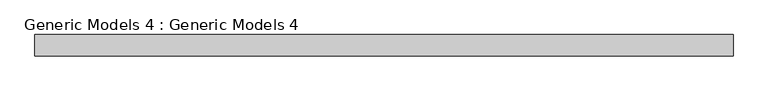
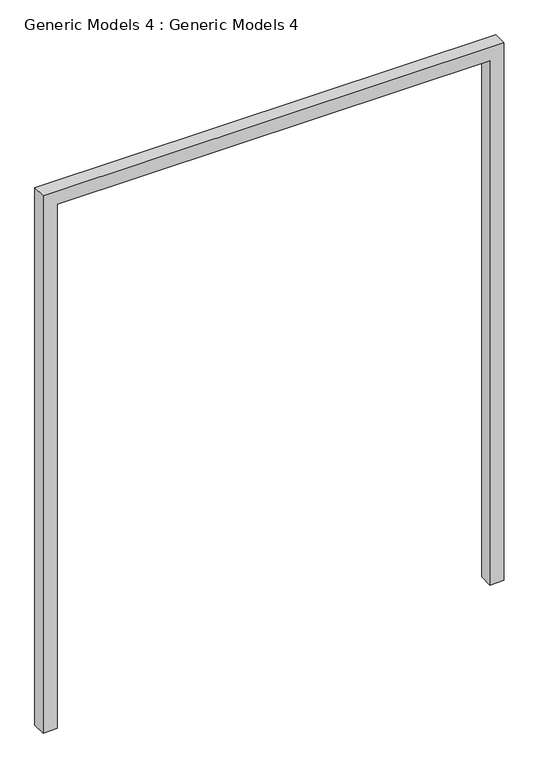
"""IFC4 building model written with IfcOpenShell, lengths in millimetres: proxy geometry, Generic Models 4 : Generic Models 4."""

from ifc_helpers import new_model, si_unit, frame, origin, place, context, project, spatial, polyline, outline, extrude, source, transform, mapped, element, save


def generic_models_4_generic_models_4_090447d9(model_context):
    return source(origin(), model_context, "Body", "SweptSolid", [
        extrude(outline(polyline([(5201.6, -5076.4678816), (3200.4, -5076.4678816), (3200.4, -5025.6678816), (5252.4, -5025.6678816), (5252.4, -6691.2678816), (3200.4, -6691.2678816), (3200.4, -6640.4678816), (5201.6, -6640.4678816), (5201.6, -5076.4678816)])), frame((0.0, 2581.1030358, 0.0), z_axis=(0.0, 1.0, 0.0), x_axis=(0.0, 0.0, 1.0)), (0.0, 0.0, 1.0), 50.8),
    ])


if __name__ == "__main__":
    model = new_model("IFC4")
    model_context = context("Model", 3, world=origin())
    ifc_project = project(units=[si_unit("LENGTHUNIT", "METRE", prefix="MILLI")], contexts=[model_context])
    site = spatial("IfcSite", under=ifc_project)
    building = spatial("IfcBuilding", under=site)
    placement = place(None, origin())
    generic_models_4_generic_models_4_shape = generic_models_4_generic_models_4_090447d9(model_context)
    element("IfcBuildingElementProxy", 1, Name="Generic Models 4 : Generic Models 4", ObjectType="Generic Models 4 : Generic Models 4", at=placement, inside=building, context=model_context, shape_type="MappedRepresentation", body=[
        mapped(generic_models_4_generic_models_4_shape, transform((0.0, 0.0, 0.0), x_axis=(1.0, 0.0, 0.0), y_axis=(0.0, 1.0, 0.0), z_axis=(0.0, 0.0, 1.0))),
    ])
    save(model, "model.ifc")

# Revit data of these elements
# Element 1 (IfcBuildingElementProxy, "Generic Models 4 : Generic Models 4")
#   Materials on its faces: "Damp-proofing"
# Materials
#   "Damp-proofing": class "Generic", colour RGB 127 127 127, transparency 0, Description = "Damp-proofing", Cost = 0
